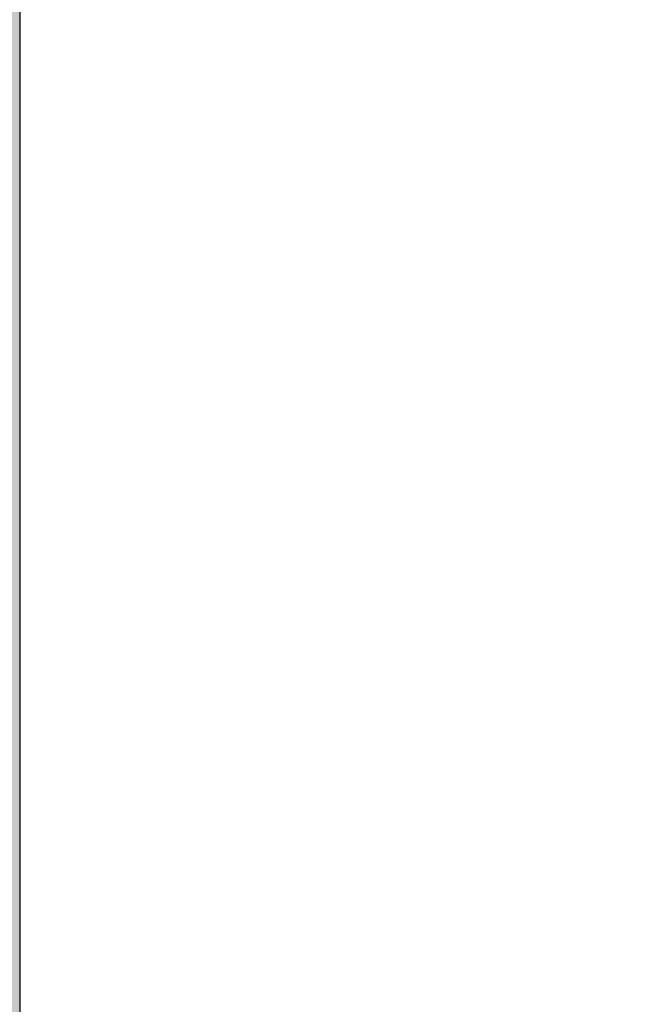
# Model space of a CAD drawing. Units: inches. Extents: x 2091 to 2899, y 967 to 2217.
# Tile 79 of 256: x 2212 to 2223, y 1114 to 1131. Entities that reach past the tile are written whole.
import ezdxf

# ---------------------------------------------------------------- set-up
doc = ezdxf.new("R2010")
doc.units = ezdxf.units.IN
doc.layers.add('A-ANNO-DIMS', color=2, linetype='Continuous', lineweight=18)
doc.layers.add('A-WALL-PATT', color=141, linetype='Continuous', lineweight=13, true_color=0xadddf7)
doc.styles.get("Standard").update_dxf_attribs({"font": 'arial.ttf'})
doc.dimstyles.new('ISO-25', dxfattribs={"dimtxt": 4, "dimasz": 4, "dimexe": 1.25, "dimexo": 0.625, "dimtad": 1, "dimdec": 0, "dimlunit": 3, "dimtxsty": 'Standard', "dimcen": 2.5, "dimadec": 0, "dimazin": 0, "dimtfac": 1, "dimtdec": 0, "dimtmove": 0, "dimatfit": 3, "dimfxl": 1, "dimarcsym": 0})

# ---------------------------------------------------------------- blocks, each defined once
blk = doc.blocks.new('*D71')
at = {"layer": 'A-ANNO-DIMS', "color": 0, "lineweight": -2, "transparency": 16777216}
for p, q in [((2212.144, 1351.294), (2212.144, 969.464)), ((2452.144, 1351.294), (2452.144, 969.464)), ((2216.144, 970.714), (2448.144, 970.714))]:
    blk.add_line(p, q, dxfattribs=at)
at = {"layer": 'A-ANNO-DIMS', "color": 0, "transparency": 16777216}
for points in [[(2216.144, 971.381), (2216.144, 970.048), (2212.144, 970.714)], [(2448.144, 971.381), (2448.144, 970.048), (2452.144, 970.714)]]:
    blk.add_solid(points, dxfattribs=at)
at = {"layer": 'Defpoints', "color": 0, "transparency": 16777216}
for p in [(2212.144, 1351.919), (2452.144, 1351.919), (2452.144, 970.714)]:
    blk.add_point(p, dxfattribs=at)
at = {"layer": 'A-ANNO-DIMS', "color": 0, "transparency": 16777216, "insert": (2332.144, 973.382), "char_height": 4, "attachment_point": 5}
blk.add_mtext('20\'-0"', dxfattribs=at)
blk = doc.blocks.new('*D75')
at = {"layer": 'A-ANNO-DIMS', "color": 0, "lineweight": -2, "transparency": 16777216}
for p, q in [((2212.144, 1274.794), (2212.144, 969.464)), ((2308.144, 1274.794), (2308.144, 969.464)), ((2216.144, 970.714), (2304.144, 970.714))]:
    blk.add_line(p, q, dxfattribs=at)
at = {"layer": 'A-ANNO-DIMS', "color": 0, "transparency": 16777216}
for points in [[(2216.144, 971.381), (2216.144, 970.048), (2212.144, 970.714)], [(2304.144, 971.381), (2304.144, 970.048), (2308.144, 970.714)]]:
    blk.add_solid(points, dxfattribs=at)
at = {"layer": 'Defpoints', "color": 0, "transparency": 16777216}
for p in [(2212.144, 1275.419), (2308.144, 1275.419), (2308.144, 970.714)]:
    blk.add_point(p, dxfattribs=at)
at = {"layer": 'A-ANNO-DIMS', "color": 0, "transparency": 16777216, "insert": (2260.144, 973.382), "char_height": 4, "attachment_point": 5}
blk.add_mtext('8\'-0"', dxfattribs=at)
blk = doc.blocks.new('*D91')
at = {"layer": 'A-ANNO-DIMS', "color": 0, "lineweight": -2, "transparency": 16777216}
for p, q in [((2211.651, 1152.247), (2098.311, 1152.247)), ((2099.561, 1103.919), (2099.561, 1148.247)), ((2211.519, 1099.919), (2098.311, 1099.919))]:
    blk.add_line(p, q, dxfattribs=at)
at = {"layer": 'A-ANNO-DIMS', "color": 0, "transparency": 16777216}
for points in [[(2098.895, 1148.247), (2100.228, 1148.247), (2099.561, 1152.247)], [(2098.895, 1103.919), (2100.228, 1103.919), (2099.561, 1099.919)]]:
    blk.add_solid(points, dxfattribs=at)
at = {"layer": 'Defpoints', "color": 0, "transparency": 16777216}
for p in [(2099.561, 1152.247), (2212.276, 1152.247), (2212.144, 1099.919)]:
    blk.add_point(p, dxfattribs=at)
at = {"layer": 'A-ANNO-DIMS', "color": 0, "transparency": 16777216, "insert": (2096.868, 1126.083), "char_height": 4, "attachment_point": 5, "rotation": 90}
blk.add_mtext('4\'-4 1/2"', dxfattribs=at)

msp = doc.modelspace()

# ---------------------------------------------------------------- hatches: boundary and pattern name
at = {"layer": 'A-WALL-PATT'}
h = msp.add_hatch(color=256, dxfattribs=at)
h.dxf.hatch_style = 1
h.paths.add_polyline_path([(2803.144, 2050.919), (2203.144, 2050.919), (2203.144, 1090.919), (2803.144, 1090.919)])
h.paths.add_polyline_path([(2635.799, 1147.54), (2674.524, 1147.54, 0.376086), (2678.53, 1152.88), (2678.53, 1159.556, 0.333335), (2674.524, 1163.562), (2674.524, 1163.562), (2674.524, 1192.934), (2635.806, 1192.934), (2597.088, 1192.934), (2597.088, 1163.562, 0.333335), (2593.082, 1159.556), (2593.082, 1152.88, 0.376086), (2597.088, 1147.54)], flags=0)
h.paths.add_polyline_path([(2436.01, 1278.241, 0.000483), (2435.953, 1278.215, -0.001328), (2435.936, 1278.112, -0.001711), (2436.116, 1278.041, 0.002185)], flags=0)
h.paths.add_polyline_path([(2794.144, 1143.419), (2794.144, 1347.419), (2543.37, 1347.419), (2543.37, 1351.919), (2794.144, 1351.919), (2794.144, 1392.714), (2793.947, 1392.714), (2793.947, 1473.537), (2794.144, 1473.537), (2794.144, 1531.919), (2650.144, 1531.919), (2650.144, 1536.419), (2794.144, 1536.419), (2794.144, 1692.419), (2609.376, 1692.419), (2609.376, 1644.419), (2604.876, 1644.419), (2604.876, 1744.919), (2609.376, 1744.919), (2609.376, 1696.919), (2794.144, 1696.919), (2794.144, 1780.919), (2609.644, 1780.919), (2493.876, 1780.919), (2493.876, 1785.419), (2609.644, 1785.419), (2794.144, 1785.419), (2794.144, 1847.939), (2793.951, 1847.939), (2793.951, 1928.762), (2794.144, 1928.762), (2794.144, 1941.419), (2614.144, 1941.419), (2614.144, 1821.419), (2609.644, 1821.419), (2609.644, 1941.419), (2392.144, 1941.419), (2392.144, 1819.919), (2387.644, 1819.919), (2387.644, 1941.419), (2212.144, 1941.419), (2212.144, 1783.919), (2392.144, 1783.919), (2392.144, 1780.919), (2212.144, 1780.919), (2212.144, 1629.419), (2387.644, 1629.419), (2387.644, 1744.919), (2392.144, 1744.919), (2392.144, 1627.919), (2317.144, 1627.919), (2317.144, 1551.419), (2317.144, 1536.419), (2459.384, 1536.419), (2459.384, 1602.396), (2463.884, 1602.396), (2463.884, 1531.919), (2456.644, 1531.919), (2456.644, 1529.919), (2452.144, 1529.919), (2452.144, 1531.919), (2312.644, 1531.919), (2312.644, 1551.419), (2306.144, 1551.419), (2306.144, 1555.919), (2308.144, 1555.919), (2308.144, 1551.419), (2312.644, 1551.419), (2312.644, 1627.919), (2212.144, 1627.919), (2212.144, 1555.919), (2270.144, 1555.919), (2270.144, 1551.419), (2212.144, 1551.419), (2212.144, 1351.919), (2272.144, 1351.919), (2272.144, 1347.419), (2212.144, 1347.419), (2212.144, 1275.419), (2308.144, 1275.419), (2308.144, 1351.919), (2452.144, 1351.919), (2452.144, 1493.919), (2456.644, 1493.919), (2456.644, 1347.419), (2312.644, 1347.419), (2312.644, 1270.919), (2212.144, 1270.919), (2212.144, 1099.919), (2281.238, 1099.919), (2282.871, 1110.914), (2282.008, 1116.997), (2278.558, 1121.42), (2268.206, 1128.056), (2272.088, 1128.056), (2273.813, 1131.927), (2279.42, 1134.692), (2285.028, 1135.245), (2287.616, 1137.457), (2288.047, 1138.01), (2289.341, 1140.775), (2291.067, 1139.669), (2292.361, 1135.245), (2295.38, 1136.904), (2296.243, 1135.798), (2297.105, 1133.033), (2300.125, 1138.01), (2303.144, 1138.01), (2304.438, 1135.798), (2303.144, 1133.586), (2306.595, 1134.692), (2307.889, 1133.033), (2310.908, 1135.245), (2313.927, 1134.139), (2315.627, 1132.427), (2308.32, 1117.55), (2290.204, 1109.808), (2288.91, 1103.172), (2289.272, 1099.919), (2434.918, 1099.919), (2431.593, 1124.788), (2429.93, 1169.553), (2430.927, 1240.52), (2435.659, 1238.186), (2437.135, 1196.554), (2438.798, 1143.973), (2442.678, 1111.998), (2446.558, 1099.919), (2794.144, 1099.919), (2794.144, 1138.919), (2548.032, 1138.919), (2548.032, 1143.419), (2548.032, 1148.819), (2546.668, 1148.032), (2528.686, 1179.179, 0.256256), (2512.032, 1148.819), (2512.032, 1143.419), (2512.032, 1138.919), (2507.532, 1138.919), (2507.532, 1143.419), (2507.532, 1148.819, 0.256256), (2490.879, 1179.179), (2472.896, 1148.032), (2471.532, 1148.819), (2471.532, 1143.419), (2467.032, 1143.419), (2467.032, 1269.946, 0.039061), (2460.91, 1273.58), (2467.032, 1273.58), (2467.032, 1286.325, 0.014511), (2465.216, 1286.762), (2467.032, 1287.053), (2467.032, 1323.419), (2471.532, 1323.419), (2471.532, 1148.819), (2489.532, 1179.996), (2490.896, 1179.208), (2490.879, 1179.179, -0.256256), (2507.532, 1148.819), (2507.532, 1143.419), (2512.032, 1143.419), (2512.032, 1148.819, -0.256256), (2528.686, 1179.179), (2528.668, 1179.208), (2530.032, 1179.996), (2548.032, 1148.819), (2548.032, 1143.419)], flags=16)
h.paths.add_polyline_path([(2607.769, 1200.945), (2607.769, 1265.031), (2597.088, 1281.052), (2619.785, 1281.052), (2627.795, 1337.127), (2635.799, 1337.127), (2643.817, 1337.127), (2651.827, 1281.052), (2674.524, 1281.052), (2663.843, 1265.031), (2663.843, 1200.945), (2635.806, 1200.945)], flags=0)
edge = h.paths.add_edge_path(flags=0)
edge.add_ellipse((13303.896, 1272.999), major_axis=(-10595.313, 0), ratio=0.84230387, start_angle=0.6282372, end_angle=0.6465541, ccw=False)
edge.add_ellipse((2711.7, 1156.853), major_axis=(2.22, 0), ratio=0.842304, start_angle=111.5352, end_angle=180.6282, ccw=False)
edge.add_ellipse((13303.156, 1272.999), major_axis=(-10593.026, 0), ratio=0.84230387, start_angle=0.5282715, end_angle=0.6465541, ccw=False)
edge.add_line((2710.765, 1175.333), (2710.13, 1175.333))
edge.add_ellipse((2710.13, 1176.58), major_axis=(1.48, 0), ratio=0.842304, start_angle=180, end_angle=270, ccw=False)
edge.add_line((2708.65, 1176.58), (2708.65, 1200.783))
edge.add_ellipse((2710.13, 1200.783), major_axis=(1.48, 0), ratio=0.842304, start_angle=90, end_angle=180, ccw=False)
edge.add_line((2710.13, 1202.029), (2710.465, 1202.029))
edge.add_ellipse((13303.156, 1272.999), major_axis=(-10593.026, 0), ratio=0.84230387, start_angle=-0.0902291, end_angle=0.3838668, ccw=False)
edge.add_ellipse((2710.13, 1290.927), major_axis=(-1.48, 0), ratio=0.842304, start_angle=0, end_angle=90, ccw=False)
edge.add_line((2708.65, 1290.927), (2708.65, 1315.13))
edge.add_ellipse((2710.13, 1315.13), major_axis=(-1.48, 0), ratio=0.842304, start_angle=-90, end_angle=0, ccw=False)
edge.add_line((2710.13, 1316.377), (2710.706, 1316.377))
edge.add_ellipse((3238.402, 1296.29), major_axis=(528.234, 0), ratio=0.8423039, start_angle=176.34957, end_angle=177.82005, ccw=False)
edge.add_ellipse((2775.063, 1071.451), major_axis=(313.308, 0), ratio=0.8423039, start_angle=102.12597, end_angle=103.78053, ccw=False)
edge.add_ellipse((2775.063, 1078.306), major_axis=(-305.303, 0), ratio=0.8423039, start_angle=-79.79046, end_angle=-77.55537, ccw=False)
edge.add_ellipse((2695.142, 1541.975), major_axis=(-250.96, 0), ratio=0.8423039, start_angle=99.25657, end_angle=102.55493)
edge.add_line((2741.41, 1334.214), (2747.133, 1337.378))
edge.add_ellipse((2747.539, 1336.857), major_axis=(-0.74, 0), ratio=0.842304, start_angle=270, end_angle=307.9331, ccw=False)
edge.add_ellipse((2747.539, 1336.857), major_axis=(-0.74, 0), ratio=0.842304, start_angle=232.0669, end_angle=270, ccw=False)
edge.add_line((2747.945, 1337.378), (2753.667, 1334.214))
edge.add_ellipse((2799.935, 1541.975), major_axis=(250.96, 0), ratio=0.8423039, start_angle=257.44507, end_angle=260.74343)
edge.add_ellipse((2720.014, 1078.306), major_axis=(305.303, 0), ratio=0.8423039, start_angle=77.55537, end_angle=79.79046, ccw=False)
edge.add_ellipse((2720.014, 1071.451), major_axis=(-313.308, 0), ratio=0.8423039, start_angle=256.21947, end_angle=257.87403, ccw=False)
edge.add_ellipse((2256.676, 1296.29), major_axis=(-528.234, 0), ratio=0.8423039, start_angle=182.17995, end_angle=183.65043, ccw=False)
edge.add_line((2784.371, 1316.377), (2784.947, 1316.377))
edge.add_ellipse((2784.947, 1315.13), major_axis=(1.48, 0), ratio=0.842304, start_angle=0, end_angle=90, ccw=False)
edge.add_line((2786.427, 1315.13), (2786.427, 1290.927))
edge.add_ellipse((2784.947, 1290.927), major_axis=(1.48, 0), ratio=0.842304, start_angle=270, end_angle=360, ccw=False)
edge.add_ellipse((-7808.079, 1272.999), major_axis=(10593.026, 0), ratio=0.84230387, start_angle=-0.3838668, end_angle=0.0902291, ccw=False)
edge.add_line((2784.612, 1202.029), (2784.947, 1202.029))
edge.add_ellipse((2784.947, 1200.783), major_axis=(1.48, 0), ratio=0.842304, start_angle=0, end_angle=90, ccw=False)
edge.add_line((2786.427, 1200.783), (2786.427, 1176.58))
edge.add_ellipse((2784.947, 1176.58), major_axis=(-1.48, 0), ratio=0.842304, start_angle=90, end_angle=180, ccw=False)
edge.add_line((2784.947, 1175.333), (2784.313, 1175.333))
edge.add_ellipse((-7808.079, 1272.999), major_axis=(10593.026, 0), ratio=0.84230387, start_angle=-0.6186432, end_angle=-0.5282715, ccw=False)
edge.add_ellipse((2783.377, 1156.853), major_axis=(-2.22, 0), ratio=0.842304, start_angle=179.3718, end_angle=248.4648, ccw=False)
edge.add_ellipse((-7808.819, 1272.999), major_axis=(-10595.313, 0), ratio=0.842303866, start_angle=179.3534459, end_angle=179.3717628, ccw=False)
edge.add_ellipse((2780.297, 1153.501), major_axis=(-5.246, 0), ratio=0.842304, start_angle=90, end_angle=179.3534, ccw=False)
edge.add_line((2780.297, 1149.082), (2714.78, 1149.082))
edge.add_ellipse((2714.78, 1153.501), major_axis=(5.246, 0), ratio=0.842304, start_angle=180.6466, end_angle=270, ccw=False)
edge = h.paths.add_edge_path(flags=0)
edge.add_line((2718.187, 1151.008), (2718.187, 1170.472))
edge.add_ellipse((2721.147, 1170.472), major_axis=(-2.96, 0), ratio=0.842304, start_angle=-90, end_angle=0, ccw=False)
edge.add_line((2721.147, 1172.965), (2773.93, 1172.965))
edge.add_ellipse((2773.93, 1170.472), major_axis=(-2.96, 0), ratio=0.842304, start_angle=180, end_angle=270, ccw=False)
edge.add_line((2776.89, 1170.472), (2776.89, 1151.008))
edge.add_line((2776.89, 1151.008), (2718.187, 1151.008))
edge = h.paths.add_edge_path(flags=0)
edge.add_line((2718.187, 1180.234), (2718.187, 1199.058))
edge.add_ellipse((2747.539, 1320.399), major_axis=(147.018, 0), ratio=0.8423039, start_angle=256.40187, end_angle=283.59813)
edge.add_line((2776.89, 1199.058), (2776.89, 1180.234))
edge.add_ellipse((2747.539, 1301.575), major_axis=(147.018, 0), ratio=0.8423039, start_angle=256.40187, end_angle=283.59813, ccw=False)
edge = h.paths.add_edge_path(flags=0)
edge.add_ellipse((13303.156, 1272.999), major_axis=(-10591.546, 0), ratio=0.84230387, start_angle=0.0555943, end_angle=0.3777642, ccw=False)
edge.add_line((2711.617, 1262.722), (2715.667, 1249.495))
edge.add_ellipse((6413.892, 1241.692), major_axis=(-3698.236, 0), ratio=0.84230387, start_angle=-0.120897, end_angle=0.364076)
edge.add_line((2715.761, 1218.192), (2711.934, 1203.167))
edge = h.paths.add_edge_path(flags=0)
edge.add_line((2718.187, 1251.075), (2716.002, 1267.45))
edge.add_ellipse((2742.151, 1202.19), major_axis=(81.773, 0), ratio=0.842304, start_angle=94.27742, end_angle=111.83495, ccw=False)
edge.add_line((2737.01, 1270.931), (2758.067, 1270.931))
edge.add_ellipse((2752.926, 1202.19), major_axis=(81.773, 0), ratio=0.842304, start_angle=68.16505, end_angle=85.72258, ccw=False)
edge.add_line((2779.075, 1267.45), (2776.89, 1251.075))
edge.add_ellipse((2750.338, 1187.885), major_axis=(79.58, 0), ratio=0.842304, start_angle=67.20809, end_angle=85.12993)
edge.add_line((2756.035, 1254.744), (2739.043, 1254.744))
edge.add_ellipse((2744.739, 1187.885), major_axis=(79.58, 0), ratio=0.842304, start_angle=94.87007, end_angle=112.79191)
edge = h.paths.add_edge_path(flags=0)
edge.add_line((2783.143, 1203.167), (2779.316, 1218.192))
edge.add_ellipse((-918.815, 1241.692), major_axis=(3698.236, 0), ratio=0.84230387, start_angle=-0.364076, end_angle=0.120897)
edge.add_line((2779.41, 1249.495), (2783.46, 1262.722))
edge.add_ellipse((-7808.079, 1272.999), major_axis=(-10591.546, 0), ratio=0.84230387, start_angle=179.6222358, end_angle=179.9444057, ccw=False)
edge = h.paths.add_edge_path(flags=0)
edge.add_ellipse((2734.201, 1286.69), major_axis=(-0.357, 6.34), ratio=0.603834, start_angle=89.002, end_angle=253.6574, ccw=False)
edge.add_line((2730.369, 1286.542), (2730.369, 1301.352))
edge.add_line((2730.369, 1301.352), (2735.913, 1305.215))
edge.add_ellipse((2736.385, 1304.735), major_axis=(0.74, 0), ratio=0.842304, start_angle=90, end_angle=134.4802, ccw=False)
edge.add_line((2736.385, 1305.358), (2738.033, 1305.358))
edge.add_line((2738.033, 1305.358), (2738.033, 1307.708))
edge.add_ellipse((2794.202, 1307.708), major_axis=(56.169, 0), ratio=0.842304, start_angle=150.5614, end_angle=180, ccw=False)
edge.add_ellipse((2700.876, 1307.708), major_axis=(-56.169, 0), ratio=0.842304, start_angle=180, end_angle=209.4386, ccw=False)
edge.add_line((2757.044, 1307.708), (2757.044, 1305.358))
edge.add_line((2757.044, 1305.358), (2758.692, 1305.358))
edge.add_ellipse((2758.692, 1304.735), major_axis=(-0.74, 0), ratio=0.842304, start_angle=225.5198, end_angle=270, ccw=False)
edge.add_line((2759.164, 1305.215), (2764.708, 1301.352))
edge.add_line((2764.708, 1301.352), (2764.708, 1286.542))
edge.add_ellipse((2760.876, 1286.69), major_axis=(0.357, 6.34), ratio=0.603834, start_angle=106.3426, end_angle=270.998, ccw=False)
edge.add_line((2757.044, 1285.797), (2757.044, 1307.708))
edge.add_ellipse((2700.876, 1307.708), major_axis=(-56.169, 0), ratio=0.842304, start_angle=180, end_angle=209.4386)
edge.add_ellipse((2794.202, 1307.708), major_axis=(56.169, 0), ratio=0.842304, start_angle=150.5614, end_angle=180)
edge.add_line((2738.033, 1307.708), (2738.033, 1285.797))
h.paths.add_polyline_path([(2417.812, 1104.45), (2413.492, 1102.53), (2410.612, 1103.97), (2409.172, 1106.37), (2407.252, 1107.33), (2406.292, 1109.73), (2405.332, 1114.05), (2405.332, 1117.89), (2406.292, 1120.13), (2407.252, 1119.81), (2408.848, 1118.328), (2410.174, 1119.424), (2410.211, 1120.406), (2411.041, 1121.419), (2410.699, 1119.859), (2410.174, 1119.424), (2410.088, 1117.176), (2411.133, 1116.206), (2413.972, 1119.33), (2416.852, 1120.77), (2416.87, 1120.799), (2417.035, 1119.405), (2417.896, 1118.143), (2418.292, 1118.37), (2419.544, 1120.039), (2419.361, 1118.387), (2419.032, 1119.356), (2418.399, 1118.512), (2419.252, 1114.53), (2418.794, 1107.199)], flags=0)
h.paths.add_polyline_path([(2508.87, 1347.419), (2508.37, 1347.419), (2508.37, 1351.919), (2508.87, 1351.919)], flags=0)
h.paths.add_polyline_path([(2473.37, 1347.419), (2472.37, 1347.419), (2467.87, 1347.419), (2467.87, 1455.419), (2472.37, 1455.419), (2472.37, 1352.419), (2473.37, 1352.419)], flags=0)
h.paths.add_polyline_path([(2352.106, 1217.446), (2349.226, 1218.886), (2347.786, 1221.286), (2345.866, 1222.246), (2344.906, 1224.646), (2343.946, 1228.966), (2343.946, 1232.806), (2344.906, 1235.046), (2345.866, 1234.726), (2347.462, 1233.244), (2348.788, 1234.341), (2348.825, 1235.322), (2349.655, 1236.336), (2349.313, 1234.775), (2348.788, 1234.341), (2348.702, 1232.093), (2349.747, 1231.123), (2352.586, 1234.246), (2355.466, 1235.686), (2355.484, 1235.715), (2355.649, 1234.322), (2356.51, 1233.06), (2356.906, 1233.286), (2358.158, 1234.956), (2357.975, 1233.304), (2357.646, 1234.273), (2357.013, 1233.428), (2357.866, 1229.446), (2357.408, 1222.115), (2356.426, 1219.366)], flags=0)
h.paths.add_polyline_path([(2348.297, 1112.224), (2347.014, 1112.31), (2345.53, 1114.127), (2345.732, 1115.858), (2346.812, 1116.982), (2346.812, 1114.646), (2345.867, 1114.214), (2346.88, 1114.3)], flags=0)
h.paths.add_polyline_path([(2347.014, 1110.926), (2346.272, 1110.493), (2346.61, 1111.186)], flags=0)
h.paths.add_polyline_path([(2345.867, 1118.194), (2345.53, 1117.329), (2343.708, 1118.021), (2344.383, 1118.626)], flags=0)
h.paths.add_polyline_path([(2346.677, 1109.282), (2346.07, 1108.071), (2345.867, 1110.061)], flags=0)
h.paths.add_polyline_path([(2345.057, 1119.751), (2343.64, 1119.751), (2343.978, 1121.135)], flags=0)
h.paths.add_polyline_path([(2345.26, 1116.55), (2345.125, 1115.858), (2344.922, 1115.685), (2344.72, 1116.377)], flags=0)
h.paths.add_polyline_path([(2345.665, 1112.31), (2345.462, 1111.532), (2344.045, 1111.964), (2344.652, 1112.57)], flags=0)
h.paths.add_polyline_path([(2345.192, 1113.349), (2344.45, 1113.868), (2344.72, 1114.387)], flags=0)
h.paths.add_polyline_path([(2344.652, 1116.809), (2344.18, 1115.685), (2344.652, 1115.339), (2343.91, 1114.906), (2343.033, 1115.944), (2343.64, 1116.463)], flags=0)
h.paths.add_polyline_path([(2345.867, 1106.686), (2344.99, 1105.562), (2344.517, 1106.6)], flags=0)
h.paths.add_polyline_path([(2344.855, 1110.061), (2344.517, 1109.282), (2344.113, 1109.715)], flags=0)
h.paths.add_polyline_path([(2344.045, 1113.522), (2343.438, 1113.089), (2342.763, 1113.954)], flags=0)
h.paths.add_polyline_path([(2344.315, 1111.012), (2342.965, 1110.32), (2342.965, 1111.099)], flags=0)
h.paths.add_polyline_path([(2345.125, 1104.697), (2344.585, 1103.745), (2344.45, 1104.264)], flags=0)
h.paths.add_polyline_path([(2342.83, 1121.222), (2341.75, 1120.53), (2340.536, 1121.049), (2340.131, 1121.828), (2340.671, 1122.952), (2341.143, 1121.828), (2341.615, 1122.001)], flags=0)
h.paths.add_polyline_path([(2342.965, 1119.751), (2343.033, 1118.453), (2342.088, 1118.021), (2342.02, 1119.491)], flags=0)
h.paths.add_polyline_path([(2342.695, 1116.896), (2341.953, 1116.636), (2342.02, 1117.329)], flags=0)
h.paths.add_polyline_path([(2343.033, 1112.224), (2342.02, 1111.791), (2341.548, 1112.224), (2342.358, 1113.349)], flags=0)
h.paths.add_polyline_path([(2343.775, 1104.437), (2342.628, 1102.88), (2342.695, 1104.61), (2343.438, 1105.129)], flags=0)
h.paths.add_polyline_path([(2342.02, 1115.079), (2340.806, 1115.512), (2340.941, 1116.377)], flags=0)
h.paths.add_polyline_path([(2341.481, 1120.097), (2341.481, 1119.405), (2341.076, 1119.578), (2341.143, 1120.097)], flags=0)
h.paths.add_polyline_path([(2341.818, 1114.473), (2340.941, 1113.089), (2340.806, 1114.56)], flags=0)
h.paths.add_polyline_path([(2341.143, 1118.54), (2340.941, 1116.982), (2339.051, 1117.675), (2339.051, 1118.626)], flags=0)
h.paths.add_polyline_path([(2342.695, 1101.668), (2341.953, 1101.841), (2342.56, 1102.361)], flags=0)
h.paths.add_polyline_path([(2340.333, 1119.665), (2338.444, 1119.578), (2337.904, 1120.357), (2339.658, 1120.616)], flags=0)
h.paths.add_polyline_path([(2340.333, 1115.339), (2340.063, 1113.695), (2339.388, 1115.339)], flags=0)
h.paths.add_polyline_path([(2341.818, 1103.831), (2341.548, 1102.88), (2341.143, 1103.658)], flags=0)
h.paths.add_polyline_path([(2339.051, 1122.866), (2337.296, 1121.828), (2337.094, 1123.125), (2337.769, 1123.818)], flags=0)
h.paths.add_polyline_path([(2339.118, 1121.741), (2338.848, 1121.222), (2338.174, 1121.049), (2338.376, 1121.568)], flags=0)
h.paths.add_polyline_path([(2339.186, 1119.319), (2338.646, 1118.713), (2338.241, 1118.107), (2338.241, 1118.886)], flags=0)
h.paths.add_polyline_path([(2341.143, 1101.928), (2340.603, 1101.236), (2340.063, 1101.841), (2340.603, 1102.361)], flags=0)
h.paths.add_polyline_path([(2337.634, 1117.761), (2336.621, 1118.28), (2337.296, 1118.972)], flags=0)
h.paths.add_polyline_path([(2336.824, 1119.578), (2334.799, 1118.972), (2335.204, 1120.357), (2336.554, 1120.876)], flags=0)
h.paths.add_polyline_path([(2339.118, 1100.457), (2337.364, 1100.543), (2336.756, 1101.236)], flags=0)
h.paths.add_polyline_path([(2336.351, 1122.433), (2336.014, 1121.914), (2334.934, 1122.433), (2334.529, 1123.471), (2335.744, 1122.779)], flags=0)
h.paths.add_polyline_path([(2334.732, 1120.876), (2334.259, 1120.357), (2334.057, 1120.789), (2334.597, 1121.308)], flags=0)
h.paths.add_polyline_path([(2334.462, 1122.174), (2332.572, 1121.308), (2331.357, 1122.174), (2332.1, 1122.866)], flags=0)
h.paths.add_polyline_path([(2334.259, 1118.54), (2333.382, 1118.453), (2333.652, 1119.319)], flags=0)
h.paths.add_polyline_path([(2335.542, 1102.274), (2334.192, 1102.62), (2335.272, 1103.312)], flags=0)
h.paths.add_polyline_path([(2332.707, 1119.665), (2331.695, 1120.443), (2332.505, 1120.789)], flags=0)
h.paths.add_polyline_path([(2334.732, 1101.149), (2333.517, 1101.582), (2333.989, 1101.755)], flags=0)
h.paths.add_polyline_path([(2332.64, 1116.636), (2331.087, 1116.29), (2331.965, 1118.194)], flags=0)
h.paths.add_polyline_path([(2330.75, 1121.568), (2330.277, 1120.27), (2328.523, 1119.319), (2328.995, 1121.049)], flags=0)
h.paths.add_polyline_path([(2330.75, 1118.626), (2330.008, 1117.502), (2329.873, 1118.021)], flags=0)
h.paths.add_polyline_path([(2332.1, 1102.361), (2330.547, 1102.014), (2331.695, 1102.966)], flags=0)
h.paths.add_polyline_path([(2329.535, 1113.608), (2329.063, 1112.31), (2328.59, 1113.349)], flags=0)
h.paths.add_polyline_path([(2328.388, 1117.848), (2327.51, 1116.55), (2327.173, 1117.761)], flags=0)
h.paths.add_polyline_path([(2329.738, 1106.513), (2329.535, 1105.302), (2328.253, 1106.081)], flags=0)
h.paths.add_polyline_path([(2328.658, 1114.387), (2328.05, 1114.127), (2328.32, 1114.906)], flags=0)
h.paths.add_polyline_path([(2328.32, 1112.224), (2327.106, 1112.137), (2326.701, 1112.656)], flags=0)
h.paths.add_polyline_path([(2326.903, 1115.252), (2326.701, 1114.127), (2325.216, 1113.608), (2326.093, 1115.339)], flags=0)
h.paths.add_polyline_path([(2326.633, 1108.33), (2326.093, 1107.379), (2325.891, 1108.503), (2326.498, 1109.109)], flags=0)
h.paths.add_polyline_path([(2615.144, 1531.919), (2609.644, 1531.919), (2609.644, 1620.419), (2614.144, 1620.419), (2614.144, 1536.419), (2615.144, 1536.419)], flags=0)
h.paths.add_polyline_path([(2545.144, 1563.419), (2464.144, 1563.419), (2464.144, 1632.419), (2509.144, 1632.419), (2509.144, 1627.919), (2509.144, 1603.919), (2468.644, 1603.919), (2468.644, 1567.919), (2540.644, 1567.919), (2540.644, 1591.919), (2545.144, 1591.919)], flags=0)
h.paths.add_polyline_path([(2388.969, 1549.986), (2357.434, 1549.986), (2357.434, 1623.361), (2399.363, 1623.361), (2435.689, 1623.361), (2435.593, 1602.559), (2435.593, 1602.396), (2388.969, 1602.396)], flags=0)
h.paths.add_polyline_path([(2388.881, 1555.809), (2374.904, 1555.809), (2374.904, 1600.572), (2374.904, 1615.458), (2406.351, 1615.458), (2406.351, 1618.939), (2412.174, 1615.458), (2406.351, 1611.976), (2406.351, 1615.458), (2388.881, 1615.458)], flags=0)
h.paths.add_polyline_path([(2568.876, 1644.419), (2453.376, 1644.419), (2453.376, 1785.419), (2457.876, 1785.419), (2457.876, 1648.919), (2568.876, 1648.919)], flags=0)
h.paths.add_polyline_path([(2212.144, 1945.919), (2212.144, 2041.919), (2794.144, 2041.919), (2794.144, 1945.919)], flags=16)
h.paths.add_polyline_path([(2271.083, 1964.317), (2776.853, 1964.317), (2776.853, 2037.17), (2271.083, 2037.17)], flags=8)
h.paths.add_polyline_path([(2380.649, 1536.824), (2461.041, 1536.824), (2461.041, 1554.653), (2380.649, 1554.653)], flags=8)
h.paths.add_polyline_path([(2240.756, 1609.725), (2309.186, 1609.725), (2309.186, 1617.698), (2240.756, 1617.698)], flags=8)
h.paths.add_polyline_path([(2212.677, 1313.504), (2282.592, 1313.504), (2282.592, 1322.745), (2212.677, 1322.745)], flags=8)
h.paths.add_polyline_path([(2457.112, 1114.779), (2558.482, 1114.779), (2558.482, 1142.22), (2457.112, 1142.22)], flags=8)
h.paths.add_polyline_path([(2473.442, 1273.01), (2604.641, 1273.01), (2604.641, 1318.347), (2473.442, 1318.347)], flags=8)
h.paths.add_polyline_path([(2638.876, 1626.977), (2684.25, 1627.977), (2684.038, 1637.597), (2638.664, 1636.598)], flags=8)
h.paths.add_polyline_path([(2537.591, 1453.793), (2628.39, 1453.793), (2628.39, 1475.345), (2537.591, 1475.345)], flags=8)
h.paths.add_polyline_path([(2504.138, 1714.632), (2554.647, 1714.632), (2554.647, 1730.238), (2504.138, 1730.238)], flags=8)
h.paths.add_polyline_path([(2487.501, 1575.652), (2535.097, 1575.652), (2535.097, 1598.378), (2487.501, 1598.378)], flags=8)
h.paths.add_polyline_path([(2709.099, 1735.71), (2740.017, 1735.71), (2740.017, 1749.938), (2709.099, 1749.938)], flags=8)
h.paths.add_polyline_path([(2442.438, 1792.172), (2564.729, 1792.172), (2564.729, 1842), (2442.438, 1842)], flags=8)
h.paths.add_polyline_path([(2655.816, 1809.644), (2789.52, 1806.694), (2790.085, 1832.292), (2656.381, 1835.242)], flags=8)
h.paths.add_polyline_path([(2234.843, 1797.72), (2368.593, 1794.769), (2369.161, 1820.504), (2235.411, 1823.455)], flags=8)
h.paths.add_polyline_path([(2245.138, 1644.006), (2398.428, 1640.624), (2398.995, 1666.325), (2245.706, 1669.707)], flags=8)
h.paths.add_polyline_path([(2306.143, 1431.169), (2413.768, 1428.794), (2414.333, 1454.392), (2306.708, 1456.766)], flags=8)
h.paths.add_polyline_path([(2306.835, 1458.233), (2393.38, 1456.323), (2393.933, 1481.354), (2307.387, 1483.264)], flags=8)

# ---------------------------------------------------------------- dimensions: what is measured, and where the dimension line sits
at = {"layer": 'A-ANNO-DIMS'}
for base, p1, p2, picture, middle in [((2452.144, 970.714), (2212.144, 1351.919), (2452.144, 1351.919), '*D71', (2332.144, 973.382)), ((2308.144, 970.714), (2212.144, 1275.419), (2308.144, 1275.419), '*D75', (2260.144, 973.382))]:
    dim = msp.add_linear_dim(base=base, p1=p1, p2=p2, dimstyle='ISO-25', override={"dimdec": 1, "dimlfac": 1, "dimrnd": 0, "dimzin": 1, "dimdsep": 46, "dimlunit": 4, "dimfrac": 2}, dxfattribs=at)
    dim.commit()
    dim.dimension.update_dxf_attribs({"geometry": picture, "text_midpoint": middle})
dim = msp.add_linear_dim(base=(2099.561, 1152.247), p1=(2212.144, 1099.919), p2=(2212.276, 1152.247), angle=90, dimstyle='ISO-25', override={"dimdec": 1, "dimlfac": 1, "dimrnd": 0, "dimzin": 1, "dimdsep": 46, "dimlunit": 4, "dimfrac": 2}, dxfattribs=at)
dim.commit()
dim.dimension.update_dxf_attribs({"geometry": '*D91', "text_midpoint": (2096.868, 1126.083)})

doc.saveas('drawing.dxf')
